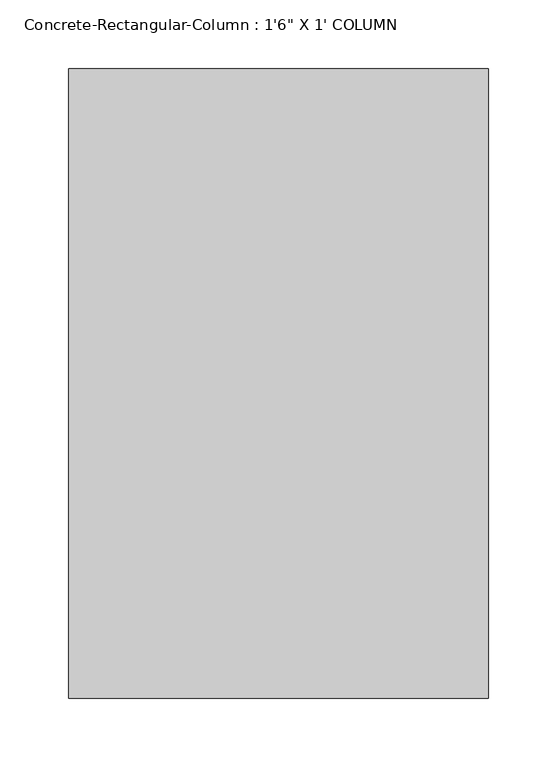
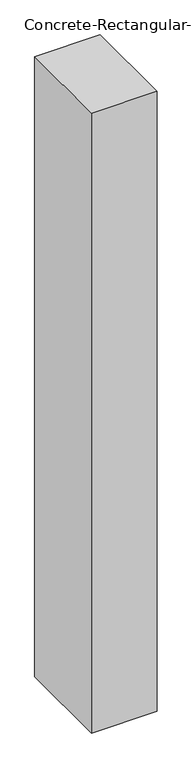
"""IFC4 building model written with IfcOpenShell, lengths in millimetres: column geometry."""

from ifc_helpers import new_model, si_unit, frame, origin, place, context, project, spatial, polyline, outline, extrude, source, transform, mapped, element, save


def column_ab9bb308(model_context):
    return source(origin(), model_context, "Body", "SweptSolid", [
        extrude(outline(polyline([(152.4, 228.6), (152.4, -228.6), (-152.4, -228.6), (-152.4, 228.6), (152.4, 228.6)])), frame((0.0, 0.0, 9448.8), z_axis=(0.0, 0.0, 1.0), x_axis=(1.0, 0.0, 0.0)), (0.0, 0.0, 1.0), 3048.0),
    ])


if __name__ == "__main__":
    model = new_model("IFC4")
    model_context = context("Model", 3, world=origin())
    ifc_project = project(units=[si_unit("LENGTHUNIT", "METRE", prefix="MILLI")], contexts=[model_context])
    site = spatial("IfcSite", under=ifc_project)
    building = spatial("IfcBuilding", under=site)
    placement = place(None, origin())
    column_shape = column_ab9bb308(model_context)
    element("IfcColumn", 1, ObjectType="Concrete-Rectangular-Column : 1'6\" X 1' COLUMN", at=placement, inside=building, context=model_context, shape_type="MappedRepresentation", body=[
        mapped(column_shape, transform((0.0, 0.0, 0.0), x_axis=(1.0, 0.0, 0.0), y_axis=(0.0, 1.0, 0.0), z_axis=(0.0, 0.0, 1.0))),
    ])
    save(model, "model.ifc")

# Revit data of these elements
# Type "Concrete-Rectangular-Column : 1'6\" X 1' COLUMN"
#   Assembly Code = "B10"
#   b = 1' - 0"
#   h = 1' - 6"
#   Structural Material [instance default] = Concrete, Cast-in-Place gray
# Element 1 (IfcColumn, "Concrete-Rectangular-Column : 1'6\" X 1' COLUMN")
#   Structural Material = WARM BEIGE COLOUR
#   Materials on its faces: "WARM BEIGE COLOUR"
# Materials
#   "Concrete, Cast-in-Place gray": class "Concrete", colour RGB 192 192 192, transparency 0, Description = "Cast-in-place concrete", Cost = 0
#   "WARM BEIGE COLOUR": class "Generic", colour RGB 120 120 120, transparency 0, Cost = 0
